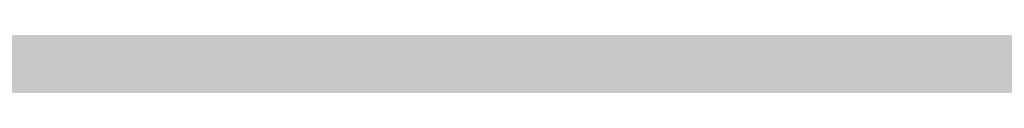
# Model space of a CAD drawing. Units: inches. Extents: x 2091 to 2899, y 967 to 2217.
# Tile 229 of 256: x 2203.4104 to 2203.7172, y 1152.2605 to 1152.274. Entities that reach past the tile are written whole.
import ezdxf

# ---------------------------------------------------------------- set-up
doc = ezdxf.new("R2010")
doc.units = ezdxf.units.IN
doc.layers.add('A-WALL-PATT', color=141, linetype='Continuous', lineweight=13, true_color=0xadddf7)

msp = doc.modelspace()

# ---------------------------------------------------------------- hatches: boundary and pattern name
at = {"layer": 'A-WALL-PATT'}
h = msp.add_hatch(color=256, dxfattribs=at)
h.dxf.hatch_style = 1
h.paths.add_polyline_path([(2803.1436, 2050.91906), (2203.1436, 2050.91906), (2203.1436, 1090.91906), (2803.1436, 1090.91906)])
h.paths.add_polyline_path([(2635.79885, 1147.54046), (2674.52405, 1147.54046, 0.376086), (2678.52967, 1152.8802), (2678.52967, 1159.55647, 0.333335), (2674.52432, 1163.56185), (2674.52432, 1163.56185), (2674.52432, 1192.93439), (2635.80597, 1192.93439), (2597.08762, 1192.93439), (2597.08762, 1163.56185, 0.333335), (2593.08228, 1159.55647), (2593.08228, 1152.8802, 0.376086), (2597.08789, 1147.54046)], flags=0)
h.paths.add_polyline_path([(2436.01043, 1278.24078, 0.000483), (2435.95264, 1278.21503, -0.001328), (2435.93563, 1278.11169, -0.001711), (2436.11644, 1278.04076, 0.002185)], flags=0)
h.paths.add_polyline_path([(2794.1436, 1143.41906), (2794.1436, 1347.41906), (2543.37017, 1347.41906), (2543.37017, 1351.91906), (2794.1436, 1351.91906), (2794.1436, 1392.71355), (2793.9474, 1392.71355), (2793.9474, 1473.5369), (2794.1436, 1473.5369), (2794.1436, 1531.91906), (2650.1436, 1531.91906), (2650.1436, 1536.41906), (2794.1436, 1536.41906), (2794.1436, 1692.41906), (2609.37561, 1692.41906), (2609.37561, 1644.41906), (2604.87561, 1644.41906), (2604.87561, 1744.91906), (2609.37561, 1744.91906), (2609.37561, 1696.91906), (2794.1436, 1696.91906), (2794.1436, 1780.91906), (2609.6436, 1780.91906), (2493.87561, 1780.91906), (2493.87561, 1785.41906), (2609.6436, 1785.41906), (2794.1436, 1785.41906), (2794.1436, 1847.93882), (2793.95122, 1847.93882), (2793.95122, 1928.76217), (2794.1436, 1928.76217), (2794.1436, 1941.41906), (2614.1436, 1941.41906), (2614.1436, 1821.41906), (2609.6436, 1821.41906), (2609.6436, 1941.41906), (2392.1436, 1941.41906), (2392.1436, 1819.91906), (2387.6436, 1819.91906), (2387.6436, 1941.41906), (2212.1436, 1941.41906), (2212.1436, 1783.91906), (2392.1436, 1783.91906), (2392.1436, 1780.91906), (2212.1436, 1780.91906), (2212.1436, 1629.41906), (2387.6436, 1629.41906), (2387.6436, 1744.91906), (2392.1436, 1744.91906), (2392.1436, 1627.91906), (2317.1436, 1627.91906), (2317.1436, 1551.41906), (2317.1436, 1536.41906), (2459.38359, 1536.41906), (2459.38359, 1602.39648), (2463.88359, 1602.39648), (2463.88359, 1531.91906), (2456.6436, 1531.91906), (2456.6436, 1529.91906), (2452.1436, 1529.91906), (2452.1436, 1531.91906), (2312.6436, 1531.91906), (2312.6436, 1551.41906), (2306.1436, 1551.41906), (2306.1436, 1555.91906), (2308.1436, 1555.91906), (2308.1436, 1551.41906), (2312.6436, 1551.41906), (2312.6436, 1627.91906), (2212.1436, 1627.91906), (2212.1436, 1555.91906), (2270.1436, 1555.91906), (2270.1436, 1551.41906), (2212.1436, 1551.41906), (2212.1436, 1351.91906), (2272.1436, 1351.91906), (2272.1436, 1347.41906), (2212.1436, 1347.41906), (2212.1436, 1275.41906), (2308.1436, 1275.41906), (2308.1436, 1351.91906), (2452.1436, 1351.91906), (2452.1436, 1493.91906), (2456.6436, 1493.91906), (2456.6436, 1347.41906), (2312.6436, 1347.41906), (2312.6436, 1270.91906), (2212.1436, 1270.91906), (2212.1436, 1099.91906), (2281.23752, 1099.91906), (2282.87104, 1110.9138), (2282.00834, 1116.9966), (2278.55774, 1121.4204), (2268.20564, 1128.0562), (2272.08764, 1128.0562), (2273.81294, 1131.927), (2279.42034, 1134.6919), (2285.02784, 1135.2449), (2287.61584, 1137.4568), (2288.04714, 1138.0098), (2289.34114, 1140.7747), (2291.06654, 1139.6687), (2292.36054, 1135.2449), (2295.37984, 1136.9038), (2296.24254, 1135.7979), (2297.10524, 1133.033), (2300.12464, 1138.0098), (2303.14394, 1138.0098), (2304.43794, 1135.7979), (2303.14394, 1133.586), (2306.59464, 1134.6919), (2307.88874, 1133.033), (2310.90804, 1135.2449), (2313.92744, 1134.1389), (2315.62686, 1132.4271), (2308.32004, 1117.5496), (2290.20384, 1109.8079), (2288.90984, 1103.1721), (2289.27231, 1099.91906), (2434.91823, 1099.91906), (2431.59323, 1124.78806), (2429.93023, 1169.55306), (2430.92718, 1240.51969), (2435.65893, 1238.18613), (2437.13523, 1196.55406), (2438.79823, 1143.97306), (2442.67823, 1111.99806), (2446.55823, 1099.91906), (2794.1436, 1099.91906), (2794.1436, 1138.91906), (2548.03245, 1138.91906), (2548.03245, 1143.41906), (2548.03245, 1148.81906), (2546.66846, 1148.03156), (2528.68569, 1179.17862, 0.256256), (2512.03245, 1148.81906), (2512.03245, 1143.41906), (2512.03245, 1138.91906), (2507.53245, 1138.91906), (2507.53245, 1143.41906), (2507.53245, 1148.81906, 0.256256), (2490.8792, 1179.17862), (2472.89644, 1148.03156), (2471.53245, 1148.81906), (2471.53245, 1143.41906), (2467.03245, 1143.41906), (2467.03245, 1269.94579, 0.039061), (2460.90999, 1273.58006), (2467.03245, 1273.58006), (2467.03245, 1286.32536, 0.014511), (2465.21619, 1286.76191), (2467.03245, 1287.05258), (2467.03245, 1323.41906), (2471.53245, 1323.41906), (2471.53245, 1148.81906), (2489.53245, 1179.99597), (2490.89644, 1179.20847), (2490.8792, 1179.17862, -0.256256), (2507.53245, 1148.81906), (2507.53245, 1143.41906), (2512.03245, 1143.41906), (2512.03245, 1148.81906, -0.256256), (2528.68569, 1179.17862), (2528.66846, 1179.20847), (2530.03245, 1179.99597), (2548.03245, 1148.81906), (2548.03245, 1143.41906)], flags=16)
h.paths.add_polyline_path([(2607.76855, 1200.94508), (2607.76855, 1265.03063), (2597.08762, 1281.05201), (2619.78459, 1281.05201), (2627.79528, 1337.12686), (2635.79885, 1337.12686), (2643.81666, 1337.12686), (2651.82736, 1281.05201), (2674.52432, 1281.05201), (2663.8434, 1265.03063), (2663.8434, 1200.94508), (2635.80597, 1200.94508)], flags=0)
edge = h.paths.add_edge_path(flags=0)
edge.add_ellipse((13303.89622, 1272.99872), major_axis=(-10595.31304, 0), ratio=0.84230387009, start_angle=0.628237219, end_angle=0.6465541, ccw=False)
edge.add_ellipse((2711.70045, 1156.85268), major_axis=(2.21977, 0), ratio=0.8423039, start_angle=111.53524, end_angle=180.62824, ccw=False)
edge.add_ellipse((13303.15629, 1272.99872), major_axis=(-10593.02631, 0), ratio=0.84230386954, start_angle=0.528271472, end_angle=0.646554097, ccw=False)
edge.add_line((2710.7646, 1175.3333), (2710.12999, 1175.3333))
edge.add_ellipse((2710.12999, 1176.57978), major_axis=(1.47985, 0), ratio=0.8423039, start_angle=180, end_angle=270, ccw=False)
edge.add_line((2708.65014, 1176.57978), (2708.65014, 1200.78291))
edge.add_ellipse((2710.12999, 1200.78291), major_axis=(1.47985, 0), ratio=0.8423039, start_angle=90, end_angle=180, ccw=False)
edge.add_line((2710.12999, 1202.02939), (2710.46508, 1202.02939))
edge.add_ellipse((13303.15629, 1272.99872), major_axis=(-10593.02631, 0), ratio=0.84230386954, start_angle=-0.090229089, end_angle=0.383866779, ccw=False)
edge.add_ellipse((2710.12999, 1290.92703), major_axis=(-1.47985, 0), ratio=0.8423039, start_angle=0, end_angle=90, ccw=False)
edge.add_line((2708.65014, 1290.92703), (2708.65014, 1315.13017))
edge.add_ellipse((2710.12999, 1315.13017), major_axis=(-1.47985, 0), ratio=0.8423039, start_angle=-90, end_angle=0, ccw=False)
edge.add_line((2710.12999, 1316.37665), (2710.70631, 1316.37665))
edge.add_ellipse((3238.40172, 1296.28957), major_axis=(528.234, 0), ratio=0.84230387, start_angle=176.3495724, end_angle=177.8200497, ccw=False)
edge.add_ellipse((2775.06304, 1071.4507), major_axis=(313.30776, 0), ratio=0.84230387, start_angle=102.1259656, end_angle=103.780529, ccw=False)
edge.add_ellipse((2775.06304, 1078.3057), major_axis=(-305.30289, 0), ratio=0.84230387, start_angle=-79.790461, end_angle=-77.5553727, ccw=False)
edge.add_ellipse((2695.14177, 1541.97538), major_axis=(-250.96022, 0), ratio=0.84230387, start_angle=99.256566, end_angle=102.5549326)
edge.add_line((2741.41033, 1334.21426), (2747.13255, 1337.37848))
edge.add_ellipse((2747.53862, 1336.85748), major_axis=(-0.73992, 0), ratio=0.842304, start_angle=270, end_angle=307.93313, ccw=False)
edge.add_ellipse((2747.53862, 1336.85748), major_axis=(-0.73992, 0), ratio=0.842304, start_angle=232.06687, end_angle=270, ccw=False)
edge.add_line((2747.94469, 1337.37848), (2753.66691, 1334.21426))
edge.add_ellipse((2799.93547, 1541.97538), major_axis=(250.96022, 0), ratio=0.84230387, start_angle=257.4450674, end_angle=260.743434)
edge.add_ellipse((2720.01419, 1078.3057), major_axis=(305.30289, 0), ratio=0.84230387, start_angle=77.5553727, end_angle=79.790461, ccw=False)
edge.add_ellipse((2720.01419, 1071.4507), major_axis=(-313.30776, 0), ratio=0.84230387, start_angle=256.219471, end_angle=257.8740344, ccw=False)
edge.add_ellipse((2256.67551, 1296.28957), major_axis=(-528.234, 0), ratio=0.84230387, start_angle=182.1799503, end_angle=183.6504276, ccw=False)
edge.add_line((2784.37092, 1316.37665), (2784.94725, 1316.37665))
edge.add_ellipse((2784.94725, 1315.13017), major_axis=(1.47985, 0), ratio=0.8423039, start_angle=0, end_angle=90, ccw=False)
edge.add_line((2786.42709, 1315.13017), (2786.42709, 1290.92703))
edge.add_ellipse((2784.94725, 1290.92703), major_axis=(1.47985, 0), ratio=0.8423039, start_angle=270, end_angle=360, ccw=False)
edge.add_ellipse((-7808.07906, 1272.99872), major_axis=(10593.02631, 0), ratio=0.84230386954, start_angle=-0.383866779, end_angle=0.090229089, ccw=False)
edge.add_line((2784.61216, 1202.02939), (2784.94725, 1202.02939))
edge.add_ellipse((2784.94725, 1200.78291), major_axis=(1.47985, 0), ratio=0.8423039, start_angle=0, end_angle=90, ccw=False)
edge.add_line((2786.42709, 1200.78291), (2786.42709, 1176.57978))
edge.add_ellipse((2784.94725, 1176.57978), major_axis=(-1.47985, 0), ratio=0.8423039, start_angle=90, end_angle=180, ccw=False)
edge.add_line((2784.94725, 1175.3333), (2784.31264, 1175.3333))
edge.add_ellipse((-7808.07906, 1272.99872), major_axis=(10593.02631, 0), ratio=0.84230386954, start_angle=-0.618643196, end_angle=-0.528271472, ccw=False)
edge.add_ellipse((2783.37678, 1156.85268), major_axis=(-2.21977, 0), ratio=0.8423039, start_angle=179.37176, end_angle=248.46476, ccw=False)
edge.add_ellipse((-7808.81898, 1272.99872), major_axis=(-10595.31304, 0), ratio=0.84230386576, start_angle=179.353445923, end_angle=179.371762803, ccw=False)
edge.add_ellipse((2780.2973, 1153.50079), major_axis=(-5.24643, 0), ratio=0.8423039, start_angle=90, end_angle=179.35345, ccw=False)
edge.add_line((2780.2973, 1149.08171), (2714.77993, 1149.08171))
edge.add_ellipse((2714.77993, 1153.50079), major_axis=(5.24643, 0), ratio=0.8423039, start_angle=180.64655, end_angle=270, ccw=False)
edge = h.paths.add_edge_path(flags=0)
edge.add_line((2718.18737, 1151.00783), (2718.18737, 1170.47236))
edge.add_ellipse((2721.14706, 1170.47236), major_axis=(-2.95969, 0), ratio=0.8423039, start_angle=-90, end_angle=0, ccw=False)
edge.add_line((2721.14706, 1172.96532), (2773.93017, 1172.96532))
edge.add_ellipse((2773.93017, 1170.47236), major_axis=(-2.95969, 0), ratio=0.8423039, start_angle=180, end_angle=270, ccw=False)
edge.add_line((2776.88987, 1170.47236), (2776.88987, 1151.00783))
edge.add_line((2776.88987, 1151.00783), (2718.18737, 1151.00783))
edge = h.paths.add_edge_path(flags=0)
edge.add_line((2718.18737, 1180.23415), (2718.18737, 1199.05783))
edge.add_ellipse((2747.53862, 1320.39864), major_axis=(147.01792, 0), ratio=0.84230387, start_angle=256.4018653, end_angle=283.5981347)
edge.add_line((2776.88987, 1199.05783), (2776.88987, 1180.23415))
edge.add_ellipse((2747.53862, 1301.57496), major_axis=(147.01792, 0), ratio=0.84230387, start_angle=256.4018653, end_angle=283.5981347, ccw=False)
edge = h.paths.add_edge_path(flags=0)
edge.add_ellipse((13303.15629, 1272.99872), major_axis=(-10591.54646, 0), ratio=0.84230386955, start_angle=0.055594314, end_angle=0.377764194, ccw=False)
edge.add_line((2711.61686, 1262.72171), (2715.66741, 1249.4954))
edge.add_ellipse((6413.89196, 1241.69192), major_axis=(-3698.23616, 0), ratio=0.8423038695, start_angle=-0.12089737, end_angle=0.36407635)
edge.add_line((2715.76104, 1218.19245), (2711.93431, 1203.16736))
edge = h.paths.add_edge_path(flags=0)
edge.add_line((2718.18737, 1251.07457), (2716.00249, 1267.45044))
edge.add_ellipse((2742.15117, 1202.18954), major_axis=(81.77258, 0), ratio=0.84230387, start_angle=94.277421, end_angle=111.8349538, ccw=False)
edge.add_line((2737.00975, 1270.93063), (2758.06748, 1270.93063))
edge.add_ellipse((2752.92606, 1202.18954), major_axis=(81.77258, 0), ratio=0.84230387, start_angle=68.1650462, end_angle=85.722579, ccw=False)
edge.add_line((2779.07475, 1267.45044), (2776.88987, 1251.07457))
edge.add_ellipse((2750.33806, 1187.88536), major_axis=(79.57966, 0), ratio=0.84230387, start_angle=67.2080851, end_angle=85.1299304)
edge.add_line((2756.03466, 1254.74366), (2739.04258, 1254.74366))
edge.add_ellipse((2744.73917, 1187.88536), major_axis=(79.57966, 0), ratio=0.84230387, start_angle=94.8700696, end_angle=112.7919149)
edge = h.paths.add_edge_path(flags=0)
edge.add_line((2783.14293, 1203.16736), (2779.31619, 1218.19245))
edge.add_ellipse((-918.81473, 1241.69192), major_axis=(3698.23616, 0), ratio=0.8423038695, start_angle=-0.36407635, end_angle=0.12089737)
edge.add_line((2779.40983, 1249.4954), (2783.46037, 1262.72171))
edge.add_ellipse((-7808.07906, 1272.99872), major_axis=(-10591.54646, 0), ratio=0.84230386954, start_angle=179.622235806, end_angle=179.944405687, ccw=False)
edge = h.paths.add_edge_path(flags=0)
edge.add_ellipse((2734.20089, 1286.69044), major_axis=(-0.35661, 6.34008), ratio=0.6038336, start_angle=89.002014, end_angle=253.657408, ccw=False)
edge.add_line((2730.369, 1286.54181), (2730.369, 1301.35198))
edge.add_line((2730.369, 1301.35198), (2735.91331, 1305.2148))
edge.add_ellipse((2736.38492, 1304.73456), major_axis=(0.73992, 0), ratio=0.842304, start_angle=90, end_angle=134.48021, ccw=False)
edge.add_line((2736.38492, 1305.3578), (2738.03278, 1305.3578))
edge.add_line((2738.03278, 1305.3578), (2738.03278, 1307.70793))
edge.add_ellipse((2794.20164, 1307.70793), major_axis=(56.16886, 0), ratio=0.84230387, start_angle=150.56143, end_angle=180, ccw=False)
edge.add_ellipse((2700.87559, 1307.70793), major_axis=(-56.16886, 0), ratio=0.84230387, start_angle=180, end_angle=209.43857, ccw=False)
edge.add_line((2757.04445, 1307.70793), (2757.04445, 1305.3578))
edge.add_line((2757.04445, 1305.3578), (2758.69232, 1305.3578))
edge.add_ellipse((2758.69232, 1304.73456), major_axis=(-0.73992, 0), ratio=0.842304, start_angle=225.51979, end_angle=270, ccw=False)
edge.add_line((2759.16392, 1305.2148), (2764.70823, 1301.35198))
edge.add_line((2764.70823, 1301.35198), (2764.70823, 1286.54181))
edge.add_ellipse((2760.87634, 1286.69044), major_axis=(0.35661, 6.34008), ratio=0.6038336, start_angle=106.342592, end_angle=270.997986, ccw=False)
edge.add_line((2757.04445, 1285.79709), (2757.04445, 1307.70793))
edge.add_ellipse((2700.87559, 1307.70793), major_axis=(-56.16886, 0), ratio=0.84230387, start_angle=180, end_angle=209.43857)
edge.add_ellipse((2794.20164, 1307.70793), major_axis=(56.16886, 0), ratio=0.84230387, start_angle=150.56143, end_angle=180)
edge.add_line((2738.03278, 1307.70793), (2738.03278, 1285.79709))
h.paths.add_polyline_path([(2417.81227, 1104.4497), (2413.49227, 1102.5297), (2410.61227, 1103.9697), (2409.17227, 1106.3697), (2407.25227, 1107.3297), (2406.29227, 1109.7297), (2405.33227, 1114.0497), (2405.33227, 1117.8897), (2406.29227, 1120.1297), (2407.25227, 1119.8097), (2408.84832, 1118.32766), (2410.17395, 1119.42417), (2410.21127, 1120.4057), (2411.04073, 1121.41905), (2410.69927, 1119.8587), (2410.17395, 1119.42417), (2410.08845, 1117.17611), (2411.13284, 1116.20632), (2413.97227, 1119.3297), (2416.85227, 1120.7697), (2416.86972, 1120.79878), (2417.03507, 1119.40512), (2417.89621, 1118.14338), (2418.29227, 1118.3697), (2419.54445, 1120.03927), (2419.36092, 1118.38749), (2419.03211, 1119.35615), (2418.39894, 1118.51193), (2419.25227, 1114.5297), (2418.79409, 1107.19879)], flags=0)
h.paths.add_polyline_path([(2508.87017, 1347.41906), (2508.37017, 1347.41906), (2508.37017, 1351.91906), (2508.87017, 1351.91906)], flags=0)
h.paths.add_polyline_path([(2473.37017, 1347.41906), (2472.37017, 1347.41906), (2467.87017, 1347.41906), (2467.87017, 1455.41906), (2472.37017, 1455.41906), (2472.37017, 1352.41906), (2473.37017, 1352.41906)], flags=0)
h.paths.add_polyline_path([(2352.10624, 1217.4462), (2349.22624, 1218.8862), (2347.78624, 1221.2862), (2345.86624, 1222.2462), (2344.90624, 1224.6462), (2343.94624, 1228.9662), (2343.94624, 1232.8062), (2344.90624, 1235.0462), (2345.86624, 1234.7262), (2347.46229, 1233.24415), (2348.78792, 1234.34066), (2348.82524, 1235.3222), (2349.6547, 1236.33555), (2349.31324, 1234.7752), (2348.78792, 1234.34066), (2348.70242, 1232.0926), (2349.74681, 1231.12282), (2352.58624, 1234.2462), (2355.46624, 1235.6862), (2355.48369, 1235.71528), (2355.64904, 1234.32161), (2356.51018, 1233.05988), (2356.90624, 1233.2862), (2358.15842, 1234.95576), (2357.97489, 1233.30398), (2357.64608, 1234.27264), (2357.01291, 1233.42842), (2357.86624, 1229.4462), (2357.40806, 1222.11529), (2356.42624, 1219.3662)], flags=0)
h.paths.add_polyline_path([(2348.2968, 1112.22442), (2347.0138, 1112.31042), (2345.5298, 1114.12742), (2345.7318, 1115.85842), (2346.8118, 1116.98242), (2346.8118, 1114.64642), (2345.8668, 1114.21442), (2346.8798, 1114.30042)], flags=0)
h.paths.add_polyline_path([(2347.0138, 1110.92642), (2346.2718, 1110.49342), (2346.6098, 1111.18642)], flags=0)
h.paths.add_polyline_path([(2345.8668, 1118.19442), (2345.5298, 1117.32942), (2343.7078, 1118.02142), (2344.3828, 1118.62642)], flags=0)
h.paths.add_polyline_path([(2346.6768, 1109.28242), (2346.0698, 1108.07142), (2345.8668, 1110.06142)], flags=0)
h.paths.add_polyline_path([(2345.0568, 1119.75142), (2343.6398, 1119.75142), (2343.9778, 1121.13542)], flags=0)
h.paths.add_polyline_path([(2345.2598, 1116.55042), (2345.1248, 1115.85842), (2344.9218, 1115.68542), (2344.7198, 1116.37742)], flags=0)
h.paths.add_polyline_path([(2345.6648, 1112.31042), (2345.4618, 1111.53242), (2344.0448, 1111.96442), (2344.6518, 1112.57042)], flags=0)
h.paths.add_polyline_path([(2345.1918, 1113.34942), (2344.4498, 1113.86842), (2344.7198, 1114.38742)], flags=0)
h.paths.add_polyline_path([(2344.6518, 1116.80942), (2344.1798, 1115.68542), (2344.6518, 1115.33942), (2343.9098, 1114.90642), (2343.0328, 1115.94442), (2343.6398, 1116.46342)], flags=0)
h.paths.add_polyline_path([(2345.8668, 1106.68642), (2344.9898, 1105.56242), (2344.5168, 1106.60042)], flags=0)
h.paths.add_polyline_path([(2344.8548, 1110.06142), (2344.5168, 1109.28242), (2344.1128, 1109.71542)], flags=0)
h.paths.add_polyline_path([(2344.0448, 1113.52242), (2343.4378, 1113.08942), (2342.7628, 1113.95442)], flags=0)
h.paths.add_polyline_path([(2344.3148, 1111.01242), (2342.9648, 1110.32042), (2342.9648, 1111.09942)], flags=0)
h.paths.add_polyline_path([(2345.1248, 1104.69742), (2344.5848, 1103.74542), (2344.4498, 1104.26442)], flags=0)
h.paths.add_polyline_path([(2342.8298, 1121.22242), (2341.7498, 1120.53042), (2340.5358, 1121.04942), (2340.1308, 1121.82842), (2340.6708, 1122.95242), (2341.1428, 1121.82842), (2341.6148, 1122.00142)], flags=0)
h.paths.add_polyline_path([(2342.9648, 1119.75142), (2343.0328, 1118.45342), (2342.0878, 1118.02142), (2342.0198, 1119.49142)], flags=0)
h.paths.add_polyline_path([(2342.6948, 1116.89642), (2341.9528, 1116.63642), (2342.0198, 1117.32942)], flags=0)
h.paths.add_polyline_path([(2343.0328, 1112.22442), (2342.0198, 1111.79142), (2341.5478, 1112.22442), (2342.3578, 1113.34942)], flags=0)
h.paths.add_polyline_path([(2343.7748, 1104.43742), (2342.6278, 1102.88042), (2342.6948, 1104.61042), (2343.4378, 1105.12942)], flags=0)
h.paths.add_polyline_path([(2342.0198, 1115.07942), (2340.8058, 1115.51242), (2340.9408, 1116.37742)], flags=0)
h.paths.add_polyline_path([(2341.4808, 1120.09742), (2341.4808, 1119.40542), (2341.0758, 1119.57842), (2341.1428, 1120.09742)], flags=0)
h.paths.add_polyline_path([(2341.8178, 1114.47342), (2340.9408, 1113.08942), (2340.8058, 1114.56042)], flags=0)
h.paths.add_polyline_path([(2341.1428, 1118.54042), (2340.9408, 1116.98242), (2339.0508, 1117.67542), (2339.0508, 1118.62642)], flags=0)
h.paths.add_polyline_path([(2342.6948, 1101.66842), (2341.9528, 1101.84142), (2342.5598, 1102.36142)], flags=0)
h.paths.add_polyline_path([(2340.3328, 1119.66542), (2338.4438, 1119.57842), (2337.9038, 1120.35742), (2339.6578, 1120.61642)], flags=0)
h.paths.add_polyline_path([(2340.3328, 1115.33942), (2340.0628, 1113.69542), (2339.3878, 1115.33942)], flags=0)
h.paths.add_polyline_path([(2341.8178, 1103.83142), (2341.5478, 1102.88042), (2341.1428, 1103.65842)], flags=0)
h.paths.add_polyline_path([(2339.0508, 1122.86642), (2337.2958, 1121.82842), (2337.0938, 1123.12542), (2337.7688, 1123.81842)], flags=0)
h.paths.add_polyline_path([(2339.1178, 1121.74142), (2338.8478, 1121.22242), (2338.1738, 1121.04942), (2338.3758, 1121.56842)], flags=0)
h.paths.add_polyline_path([(2339.1858, 1119.31942), (2338.6458, 1118.71342), (2338.2408, 1118.10742), (2338.2408, 1118.88642)], flags=0)
h.paths.add_polyline_path([(2341.1428, 1101.92842), (2340.6028, 1101.23642), (2340.0628, 1101.84142), (2340.6028, 1102.36142)], flags=0)
h.paths.add_polyline_path([(2337.6338, 1117.76142), (2336.6208, 1118.28042), (2337.2958, 1118.97242)], flags=0)
h.paths.add_polyline_path([(2336.8238, 1119.57842), (2334.7988, 1118.97242), (2335.2038, 1120.35742), (2336.5538, 1120.87642)], flags=0)
h.paths.add_polyline_path([(2339.1178, 1100.45742), (2337.3638, 1100.54342), (2336.7558, 1101.23642)], flags=0)
h.paths.add_polyline_path([(2336.3508, 1122.43342), (2336.0138, 1121.91442), (2334.9338, 1122.43342), (2334.5288, 1123.47142), (2335.7438, 1122.77942)], flags=0)
h.paths.add_polyline_path([(2334.7318, 1120.87642), (2334.2588, 1120.35742), (2334.0568, 1120.78942), (2334.5968, 1121.30842)], flags=0)
h.paths.add_polyline_path([(2334.4618, 1122.17442), (2332.5718, 1121.30842), (2331.3568, 1122.17442), (2332.0998, 1122.86642)], flags=0)
h.paths.add_polyline_path([(2334.2588, 1118.54042), (2333.3818, 1118.45342), (2333.6518, 1119.31942)], flags=0)
h.paths.add_polyline_path([(2335.5418, 1102.27442), (2334.1918, 1102.62042), (2335.2718, 1103.31242)], flags=0)
h.paths.add_polyline_path([(2332.7068, 1119.66542), (2331.6948, 1120.44342), (2332.5048, 1120.78942)], flags=0)
h.paths.add_polyline_path([(2334.7318, 1101.14942), (2333.5168, 1101.58242), (2333.9888, 1101.75542)], flags=0)
h.paths.add_polyline_path([(2332.6398, 1116.63642), (2331.0868, 1116.29042), (2331.9648, 1118.19442)], flags=0)
h.paths.add_polyline_path([(2330.7498, 1121.56842), (2330.2768, 1120.27042), (2328.5228, 1119.31942), (2328.9948, 1121.04942)], flags=0)
h.paths.add_polyline_path([(2330.7498, 1118.62642), (2330.0078, 1117.50242), (2329.8728, 1118.02142)], flags=0)
h.paths.add_polyline_path([(2332.0998, 1102.36142), (2330.5468, 1102.01442), (2331.6948, 1102.96642)], flags=0)
h.paths.add_polyline_path([(2329.5348, 1113.60842), (2329.0628, 1112.31042), (2328.5898, 1113.34942)], flags=0)
h.paths.add_polyline_path([(2328.3878, 1117.84842), (2327.5098, 1116.55042), (2327.1728, 1117.76142)], flags=0)
h.paths.add_polyline_path([(2329.7378, 1106.51342), (2329.5348, 1105.30242), (2328.2528, 1106.08142)], flags=0)
h.paths.add_polyline_path([(2328.6578, 1114.38742), (2328.0498, 1114.12742), (2328.3198, 1114.90642)], flags=0)
h.paths.add_polyline_path([(2328.3198, 1112.22442), (2327.1058, 1112.13742), (2326.7008, 1112.65642)], flags=0)
h.paths.add_polyline_path([(2326.9028, 1115.25242), (2326.7008, 1114.12742), (2325.2158, 1113.60842), (2326.0928, 1115.33942)], flags=0)
h.paths.add_polyline_path([(2326.6328, 1108.33042), (2326.0928, 1107.37942), (2325.8908, 1108.50342), (2326.4978, 1109.10942)], flags=0)
h.paths.add_polyline_path([(2615.1436, 1531.91906), (2609.6436, 1531.91906), (2609.6436, 1620.41906), (2614.1436, 1620.41906), (2614.1436, 1536.41906), (2615.1436, 1536.41906)], flags=0)
h.paths.add_polyline_path([(2545.1436, 1563.41906), (2464.1436, 1563.41906), (2464.1436, 1632.41906), (2509.1436, 1632.41906), (2509.1436, 1627.91906), (2509.1436, 1603.91906), (2468.6436, 1603.91906), (2468.6436, 1567.91906), (2540.6436, 1567.91906), (2540.6436, 1591.91906), (2545.1436, 1591.91906)], flags=0)
h.paths.add_polyline_path([(2388.96905, 1549.98573), (2357.43418, 1549.98573), (2357.43418, 1623.36078), (2399.36278, 1623.36078), (2435.68947, 1623.36078), (2435.59255, 1602.55927), (2435.59255, 1602.39648), (2388.96905, 1602.39648)], flags=0)
h.paths.add_polyline_path([(2388.88063, 1555.80915), (2374.90443, 1555.80915), (2374.90443, 1600.57156), (2374.90443, 1615.45765), (2406.35088, 1615.45765), (2406.35088, 1618.93943), (2412.17429, 1615.45765), (2406.35088, 1611.97586), (2406.35088, 1615.45765), (2388.88063, 1615.45765)], flags=0)
h.paths.add_polyline_path([(2568.87561, 1644.41906), (2453.37561, 1644.41906), (2453.37561, 1785.41906), (2457.87561, 1785.41906), (2457.87561, 1648.91906), (2568.87561, 1648.91906)], flags=0)
h.paths.add_polyline_path([(2212.1436, 1945.91906), (2212.1436, 2041.91906), (2794.1436, 2041.91906), (2794.1436, 1945.91906)], flags=16)
h.paths.add_polyline_path([(2271.08273, 1964.31724), (2776.85297, 1964.31724), (2776.85297, 2037.16962), (2271.08273, 2037.16962)], flags=8)
h.paths.add_polyline_path([(2380.64929, 1536.82414), (2461.04081, 1536.82414), (2461.04081, 1554.65259), (2380.64929, 1554.65259)], flags=8)
h.paths.add_polyline_path([(2240.75571, 1609.72545), (2309.18583, 1609.72545), (2309.18583, 1617.6982), (2240.75571, 1617.6982)], flags=8)
h.paths.add_polyline_path([(2212.67726, 1313.5041), (2282.59152, 1313.5041), (2282.59152, 1322.74524), (2212.67726, 1322.74524)], flags=8)
h.paths.add_polyline_path([(2457.11198, 1114.77857), (2558.48158, 1114.77857), (2558.48158, 1142.21968), (2457.11198, 1142.21968)], flags=8)
h.paths.add_polyline_path([(2473.44234, 1273.01007), (2604.64123, 1273.01007), (2604.64123, 1318.34693), (2473.44234, 1318.34693)], flags=8)
h.paths.add_polyline_path([(2638.8763, 1626.97743), (2684.25037, 1627.97674), (2684.03848, 1637.59749), (2638.66442, 1636.59819)], flags=8)
h.paths.add_polyline_path([(2537.59055, 1453.79345), (2628.38955, 1453.79345), (2628.38955, 1475.34481), (2537.59055, 1475.34481)], flags=8)
h.paths.add_polyline_path([(2504.13764, 1714.6324), (2554.64719, 1714.6324), (2554.64719, 1730.23771), (2504.13764, 1730.23771)], flags=8)
h.paths.add_polyline_path([(2487.50118, 1575.65187), (2535.09712, 1575.65187), (2535.09712, 1598.37765), (2487.50118, 1598.37765)], flags=8)
h.paths.add_polyline_path([(2709.0994, 1735.71028), (2740.0166, 1735.71028), (2740.0166, 1749.93764), (2709.0994, 1749.93764)], flags=8)
h.paths.add_polyline_path([(2442.43842, 1792.17166), (2564.72884, 1792.17166), (2564.72884, 1842.00016), (2442.43842, 1842.00016)], flags=8)
h.paths.add_polyline_path([(2655.8158, 1809.64408), (2789.52014, 1806.6938), (2790.08498, 1832.29164), (2656.38064, 1835.24192)], flags=8)
h.paths.add_polyline_path([(2234.8427, 1797.72014), (2368.59285, 1794.76885), (2369.16072, 1820.50413), (2235.41056, 1823.45542)], flags=8)
h.paths.add_polyline_path([(2245.13847, 1644.00633), (2398.42773, 1640.6239), (2398.99484, 1666.32482), (2245.70557, 1669.70725)], flags=8)
h.paths.add_polyline_path([(2306.14285, 1431.16852), (2413.76831, 1428.79369), (2414.33315, 1454.39153), (2306.70768, 1456.76636)], flags=8)
h.paths.add_polyline_path([(2306.83458, 1458.23314), (2393.38048, 1456.32345), (2393.93281, 1481.35436), (2307.38691, 1483.26405)], flags=8)

doc.saveas('drawing.dxf')
